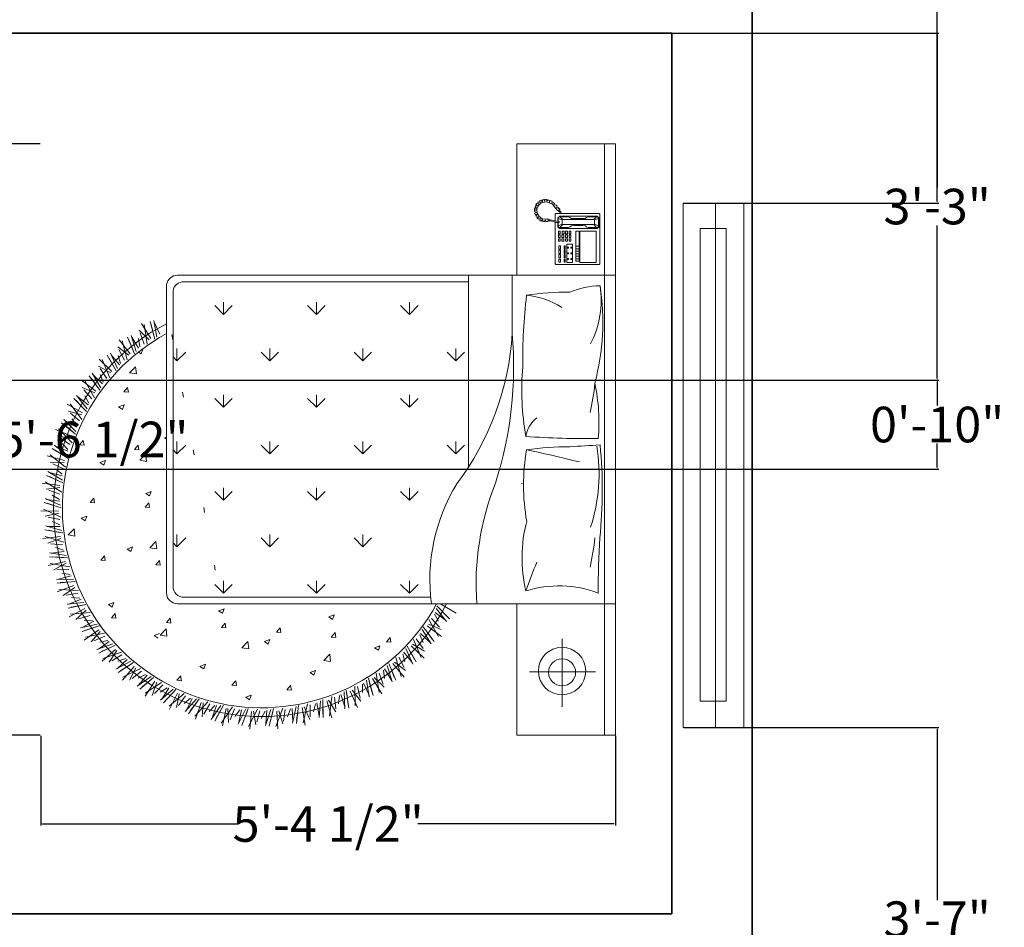
# Model space of a CAD drawing. Units: inches. Extents: x 311 to 754, y 60 to 497.
# Tile 8 of 11: x 641 to 751, y 194 to 296. Entities that reach past the tile are written whole.
import ezdxf

# ---------------------------------------------------------------- set-up
doc = ezdxf.new("R2010")
doc.units = ezdxf.units.IN
doc.header["$MEASUREMENT"] = 0
for name, color, linetype, lineweight in [('A-ANNO-DIMS', 2, 'Continuous', 18), ('A-WALL', 7, 'Continuous', 35), ('beds', 70, 'Continuous', 13), ('windows', 120, 'Continuous', 18)]:
    doc.layers.add(name, color=color, linetype=linetype, lineweight=lineweight)
doc.styles.get("Standard").update_dxf_attribs({"font": 'arial.ttf'})
doc.dimstyles.get("Standard").update_dxf_attribs({"dimtxt": 4, "dimasz": 0.18, "dimexe": 0.18, "dimexo": 0.0625, "dimgap": 0.09, "dimtad": 0, "dimtih": 1, "dimtoh": 1, "dimdec": 0, "dimrnd": 6, "dimzin": 0, "dimdsep": 46, "dimlunit": 3, "dimtxsty": 'Standard', "dimcen": 0.09, "dimadec": 0, "dimazin": 0, "dimtfac": 1, "dimtdec": 0, "dimtofl": 0, "dimtmove": 0, "dimatfit": 3, "dimfxl": 1, "dimtolj": 1, "dimtzin": 0, "dimarcsym": 0})

# ---------------------------------------------------------------- blocks, each defined once
blk = doc.blocks.new('A$C57792D97')
for p, q in [((0.6, 2.6235), (0, 2.6235)), ((0, 2.6235), (0, 2.1735)), ((2.1, 2.6235), (0.6, 2.6235)), ((0.6, 2.6235), (0.6, 0.6235)), ((0.6, 0.6235), (0.6, 2.6235)), ((0.6, 2.1735), (0.6, 2.6235)), ((2.1, 0.6235), (2.1, 2.6235)), ((2.7, 2.6235), (2.1, 2.6235)), ((2.1, 2.6235), (2.1, 2.1735)), ((2.7, 2.1735), (2.7, 2.6235)), ((0.6, 2.5735), (0, 2.5735)), ((2.1, 2.5735), (0.6, 2.5735)), ((2.7, 2.5735), (2.1, 2.5735)), ((2.4103, 2.2312), (2.4103, 2.5317)), ((2.2593, 2.3802), (2.5698, 2.3802)), ((0, 2.1735), (0.6, 2.1735)), ((1.5491, 2.1955), (1.5516, 2.1955)), ((2.1, 2.1735), (2.7, 2.1735)), ((0.6, 2.1518), (0.8661, 2.1518)), ((0.6, 1.9518), (1.4767, 1.9518)), ((0.63, 0.6535), (0.63, 1.9518)), ((0.9906, 1.8942), (0.9508, 1.934)), ((1.4149, 1.8942), (1.3751, 1.934)), ((0.9906, 1.8942), (0.9344, 1.8942)), ((0.9906, 1.8942), (0.9508, 1.8544)), ((1.4149, 1.8942), (1.3586, 1.8942)), ((1.4149, 1.8942), (1.3751, 1.8544)), ((2.142, 1.8959), (2.1018, 1.8254)), ((2.1679, 1.8652), (2.1088, 1.8077)), ((2.1584, 1.8544), (2.1201, 1.8188)), ((2.1812, 1.8524), (2.1207, 1.8046)), ((2.1749, 1.8475), (2.1394, 1.7993)), ((2.1799, 1.8155), (2.1465, 1.7971)), ((2.2066, 1.8191), (2.1664, 1.7827)), ((2.249, 1.8154), (2.1711, 1.7709)), ((2.2173, 1.8274), (2.1931, 1.7688)), ((2.2496, 1.8292), (2.2008, 1.7642)), ((2.07, 1.7793), (2.07, 0.6535)), ((2.2713, 1.7954), (2.2055, 1.7458)), ((2.283, 1.7811), (2.2169, 1.7413)), ((2.2607, 1.7859), (2.2181, 1.7554)), ((2.2761, 1.777), (2.2348, 1.7337)), ((0.7785, 1.6821), (0.7387, 1.7219)), ((1.2027, 1.6821), (1.163, 1.7219)), ((1.627, 1.6821), (1.5872, 1.7219)), ((2.0513, 1.6821), (2.0115, 1.7219)), ((2.277, 1.7446), (2.2416, 1.7306)), ((2.304, 1.7449), (2.2596, 1.7138)), ((2.3456, 1.7359), (2.2627, 1.7015)), ((2.3157, 1.7518), (2.2843, 1.6966)), ((2.3479, 1.7495), (2.2914, 1.6911)), ((2.3653, 1.7133), (2.2937, 1.6723)), ((0.7785, 1.6821), (0.7222, 1.6821)), ((0.7785, 1.6821), (0.7387, 1.6423)), ((1.2027, 1.6821), (1.1465, 1.6821)), ((1.2027, 1.6821), (1.163, 1.6423)), ((1.627, 1.6821), (1.5708, 1.6821)), ((1.627, 1.6821), (1.5872, 1.6423)), ((2.0513, 1.6821), (1.995, 1.6821)), ((2.0513, 1.6821), (2.0115, 1.6423)), ((2.3751, 1.6976), (2.3045, 1.6664)), ((2.3535, 1.7051), (2.3075, 1.6802)), ((2.3677, 1.6944), (2.3213, 1.6565)), ((2.4038, 1.6644), (2.3657, 1.6136)), ((2.3645, 1.6621), (2.3277, 1.6526)), ((2.3913, 1.659), (2.3434, 1.6337)), ((2.4314, 1.6449), (2.3449, 1.6211)), ((2.4355, 1.6581), (2.372, 1.6073)), ((2.4482, 1.62), (2.372, 1.5882)), ((2.2754, 1.598), (2.2534, 1.5939)), ((2.2736, 1.5771), (2.2535, 1.594)), ((2.2736, 1.5771), (2.2754, 1.598)), ((2.4559, 1.6032), (2.382, 1.581)), ((2.4354, 1.6134), (2.3867, 1.5944)), ((2.4482, 1.6009), (2.3974, 1.5692)), ((2.3123, 1.541), (2.2911, 1.5481)), ((2.3006, 1.5236), (2.2912, 1.5481)), ((2.3006, 1.5236), (2.3123, 1.541)), ((2.441, 1.5693), (2.4032, 1.5645)), ((2.4672, 1.5629), (2.4164, 1.5438)), ((2.5052, 1.5438), (2.4164, 1.5311)), ((2.4802, 1.5667), (2.4361, 1.5211)), ((2.5109, 1.5564), (2.4416, 1.514)), ((0.9906, 1.47), (0.9508, 1.5097)), ((1.4149, 1.47), (1.3751, 1.5097)), ((1.8391, 1.47), (1.7994, 1.5097)), ((2.5187, 1.517), (2.4392, 1.4951)), ((2.5243, 1.4994), (2.4482, 1.4867)), ((2.5052, 1.5121), (2.4545, 1.4994)), ((2.5163, 1.4981), (2.462, 1.473)), ((0.9906, 1.47), (0.9344, 1.47)), ((0.9906, 1.47), (0.9508, 1.4302)), ((1.4149, 1.47), (1.3586, 1.47)), ((1.4149, 1.47), (1.3751, 1.4302)), ((1.8391, 1.47), (1.7829, 1.47)), ((1.8391, 1.47), (1.7994, 1.4302)), ((2.5052, 1.4677), (2.4672, 1.4677)), ((2.5304, 1.458), (2.4777, 1.4454)), ((2.5438, 1.4601), (2.4943, 1.4204)), ((2.573, 1.4461), (2.4989, 1.4127)), ((2.5658, 1.4343), (2.4761, 1.4328)), ((2.5758, 1.406), (2.4942, 1.3942)), ((2.5618, 1.4028), (2.5099, 1.3966)), ((2.5791, 1.3878), (2.502, 1.3848)), ((2.571, 1.3876), (2.514, 1.3695)), ((2.5562, 1.3587), (2.5185, 1.3635)), ((2.1596, 1.3147), (2.1502, 1.3392)), ((2.1714, 1.3321), (2.1502, 1.3392)), ((2.1596, 1.3147), (2.1714, 1.3321)), ((2.2534, 1.3469), (2.2315, 1.3429)), ((2.2516, 1.326), (2.2315, 1.3429)), ((2.2516, 1.326), (2.2535, 1.347)), ((2.3632, 1.3229), (2.33, 1.319)), ((2.3584, 1.2918), (2.33, 1.319)), ((2.3584, 1.2918), (2.3632, 1.3229)), ((2.6121, 1.3181), (2.523, 1.3279)), ((2.58, 1.346), (2.5261, 1.3402)), ((2.5936, 1.3464), (2.5395, 1.3132)), ((2.6207, 1.3289), (2.5431, 1.305)), ((0.7785, 1.2578), (0.7387, 1.2976)), ((1.2027, 1.2578), (1.163, 1.2976)), ((1.627, 1.2578), (1.5872, 1.2976)), ((2.0513, 1.2578), (2.0115, 1.2976)), ((2.6185, 1.2888), (2.5361, 1.2873)), ((2.6195, 1.2703), (2.5426, 1.277)), ((2.6042, 1.2873), (2.5519, 1.2877)), ((2.6115, 1.2711), (2.5526, 1.2603)), ((0.7785, 1.2578), (0.7222, 1.2578)), ((0.7785, 1.2578), (0.7387, 1.218)), ((1.2027, 1.2578), (1.1465, 1.2578)), ((1.2027, 1.2578), (1.163, 1.218)), ((1.627, 1.2578), (1.5708, 1.2578)), ((1.627, 1.2578), (1.5872, 1.218)), ((2.0513, 1.2578), (1.995, 1.2578)), ((2.0513, 1.2578), (2.0115, 1.218)), ((2.4134, 1.2295), (2.404, 1.254)), ((2.4252, 1.2469), (2.404, 1.254)), ((2.4134, 1.2295), (2.4252, 1.2469)), ((2.5932, 1.2443), (2.5563, 1.2538)), ((2.6435, 1.197), (2.5563, 1.2178)), ((2.6152, 1.2287), (2.561, 1.2296)), ((2.6287, 1.2274), (2.5709, 1.2013)), ((2.6462, 1.1671), (2.5642, 1.176)), ((2.6534, 1.2066), (2.5734, 1.1926)), ((2.6319, 1.1675), (2.58, 1.1743)), ((2.4947, 1.1445), (2.4728, 1.1404)), ((2.4929, 1.1236), (2.4728, 1.1404)), ((2.4929, 1.1236), (2.4948, 1.1445)), ((2.6449, 1.1486), (2.5694, 1.1649)), ((2.637, 1.1504), (2.5773, 1.147)), ((2.6155, 1.1261), (2.5801, 1.1402)), ((0.9906, 1.0457), (0.9508, 1.0855)), ((1.4149, 1.0457), (1.3751, 1.0855)), ((1.8391, 1.0457), (1.7994, 1.0855)), ((2.2315, 1.0959), (2.2095, 1.0919)), ((2.2297, 1.075), (2.2096, 1.0919)), ((2.2297, 1.075), (2.2315, 1.0959)), ((2.6595, 1.0729), (2.5756, 1.1045)), ((2.6353, 1.1079), (2.5817, 1.1156)), ((2.6486, 1.1049), (2.588, 1.0862)), ((2.6705, 1.0812), (2.5894, 1.0774)), ((0.9906, 1.0457), (0.9344, 1.0457)), ((0.9906, 1.0457), (0.9508, 1.0059)), ((1.4149, 1.0457), (1.3586, 1.0457)), ((1.4149, 1.0457), (1.3751, 1.0059)), ((1.8391, 1.0457), (1.7829, 1.0457)), ((1.8391, 1.0457), (1.7994, 1.0059)), ((2.2725, 1.0206), (2.2631, 1.0451)), ((2.2842, 1.038), (2.2631, 1.0451)), ((2.2725, 1.0206), (2.2843, 1.038)), ((2.6584, 1.0429), (2.5782, 1.062)), ((2.6548, 1.0248), (2.582, 1.0503)), ((2.6442, 1.045), (2.5937, 1.0584)), ((2.6598, 0.9477), (2.5805, 0.9897)), ((2.6472, 1.0275), (2.5875, 1.0316)), ((2.6402, 0.9855), (2.588, 0.9999)), ((2.6228, 1.0061), (2.5895, 1.0244)), ((2.3053, 0.9493), (2.272, 0.9455)), ((2.3005, 0.9182), (2.2721, 0.9455)), ((2.3005, 0.9182), (2.3053, 0.9494)), ((2.5263, 0.9355), (2.5169, 0.96)), ((2.538, 0.9528), (2.5169, 0.9599)), ((2.5263, 0.9355), (2.5381, 0.9529)), ((2.655, 0.9181), (2.5778, 0.9471)), ((2.653, 0.9809), (2.5905, 0.97)), ((2.6718, 0.9546), (2.5908, 0.961)), ((2.6491, 0.9006), (2.5801, 0.9351)), ((2.6419, 0.9043), (2.5832, 0.9159)), ((2.6151, 0.8861), (2.5843, 0.9085)), ((2.6412, 0.9221), (2.5927, 0.9416)), ((0.7785, 0.8336), (0.7387, 0.8733)), ((1.2027, 0.8336), (1.163, 0.8733)), ((1.627, 0.8336), (1.5872, 0.8733)), ((2.0513, 0.8336), (2.0115, 0.8733)), ((2.4728, 0.8934), (2.4508, 0.8894)), ((2.471, 0.8725), (2.4509, 0.8894)), ((2.471, 0.8725), (2.4728, 0.8934)), ((2.6444, 0.8236), (2.571, 0.8751)), ((2.6418, 0.8573), (2.5785, 0.8543)), ((2.6297, 0.8635), (2.5797, 0.8843)), ((0.7785, 0.8336), (0.7222, 0.8336)), ((0.7785, 0.8336), (0.7387, 0.7938)), ((1.2027, 0.8336), (1.1465, 0.8336)), ((1.2027, 0.8336), (1.163, 0.7938)), ((1.627, 0.8336), (1.5708, 0.8336)), ((1.627, 0.8336), (1.5872, 0.7938)), ((2.0513, 0.8336), (1.995, 0.8336)), ((2.0513, 0.8336), (2.0115, 0.7938)), ((2.1316, 0.8117), (2.1222, 0.8362)), ((2.1433, 0.8291), (2.1222, 0.8362)), ((2.1316, 0.8117), (2.1434, 0.8291)), ((2.2095, 0.8449), (2.1876, 0.8408)), ((2.2077, 0.824), (2.1876, 0.8408)), ((2.2077, 0.824), (2.2095, 0.8449)), ((2.6359, 0.7948), (2.5629, 0.8332)), ((2.6279, 0.7781), (2.5637, 0.821)), ((2.6227, 0.8004), (2.577, 0.8259)), ((2.6572, 0.8289), (2.5776, 0.8454)), ((1.9462, 0.7963), (1.9243, 0.7923)), ((2.604, 0.7437), (2.557, 0.7707)), ((2.6212, 0.7827), (2.5644, 0.8015)), ((2.5923, 0.768), (2.5646, 0.7941)), ((1.683, 0.7477), (1.661, 0.7437)), ((2.3854, 0.7265), (2.376, 0.751)), ((2.3971, 0.7439), (2.376, 0.751)), ((2.3854, 0.7265), (2.3972, 0.7439)), ((2.6016, 0.6748), (2.534, 0.7221)), ((2.6136, 0.7023), (2.5472, 0.7626)), ((2.6269, 0.706), (2.5501, 0.7323)), ((2.6153, 0.7361), (2.552, 0.7411)), ((1.4197, 0.6992), (1.3978, 0.6951)), ((2.5549, 0.6537), (2.5307, 0.6831)), ((2.5855, 0.6646), (2.5315, 0.6905)), ((2.5915, 0.6593), (2.5332, 0.7099)), ((2.5892, 0.6821), (2.547, 0.7131)), ((0.9906, 0.6214), (0.9508, 0.6612)), ((1.1564, 0.6506), (1.1345, 0.6466)), ((1.4149, 0.6214), (1.3751, 0.6612)), ((1.8391, 0.6214), (1.7994, 0.6612)), ((2.4508, 0.6424), (2.4289, 0.6383)), ((2.449, 0.6215), (2.4289, 0.6384)), ((2.449, 0.6215), (2.4508, 0.6424)), ((2.5678, 0.5858), (2.5095, 0.654)), ((2.5737, 0.6192), (2.5116, 0.632)), ((2.5635, 0.6282), (2.5203, 0.6608)), ((2.02, 0.6035), (0.6716, 0.6035)), ((0.8932, 0.6021), (0.8712, 0.598)), ((0.9906, 0.6214), (0.9344, 0.6214)), ((0.9906, 0.6214), (0.9727, 0.6035)), ((1.4149, 0.6214), (1.3586, 0.6214)), ((1.4149, 0.6214), (1.397, 0.6035)), ((1.8391, 0.6214), (1.7829, 0.6214)), ((1.8391, 0.6214), (1.8212, 0.6035)), ((2.1875, 0.5938), (2.1656, 0.5898)), ((2.1857, 0.5729), (2.1656, 0.5898)), ((2.1857, 0.5729), (2.1876, 0.5938)), ((2.5352, 0.552), (2.4849, 0.5844)), ((2.5405, 0.546), (2.489, 0.6034)), ((2.5524, 0.5601), (2.4913, 0.6155)), ((2.541, 0.5688), (2.5031, 0.6049)), ((2.5815, 0.5878), (2.5085, 0.6236)), ((0.6417, 0.5735), (2.05, 0.5735)), ((0.8142, 0.5177), (0.8685, 0.5428)), ((1.3422, 0.5642), (1.3386, 0.5735)), ((1.3422, 0.5642), (1.3485, 0.5735)), ((1.9243, 0.5453), (1.9023, 0.5412)), ((1.9225, 0.5244), (1.9024, 0.5412)), ((1.9225, 0.5244), (1.9243, 0.5453)), ((2.2473, 0.5758), (2.2141, 0.5719)), ((2.2425, 0.5447), (2.2141, 0.572)), ((2.2445, 0.5176), (2.2351, 0.5421)), ((2.2425, 0.5447), (2.2474, 0.5758)), ((2.5078, 0.476), (2.4585, 0.551)), ((2.5088, 0.5186), (2.47, 0.5564)), ((2.5035, 0.545), (2.4831, 0.5772)), ((0.8062, 0.5164), (0.8823, 0.5291)), ((0.8118, 0.4988), (0.8913, 0.5207)), ((0.8196, 0.4594), (0.8889, 0.5018)), ((0.8253, 0.5037), (0.876, 0.5164)), ((0.8503, 0.4491), (0.8944, 0.4947)), ((1.6077, 0.4964), (1.5865, 0.5035)), ((1.596, 0.479), (1.5866, 0.5035)), ((1.596, 0.479), (1.6077, 0.4964)), ((1.661, 0.4967), (1.6391, 0.4927)), ((1.6592, 0.4758), (1.661, 0.4967)), ((1.8485, 0.5294), (1.8152, 0.5255)), ((1.8437, 0.4983), (1.8153, 0.5256)), ((1.8437, 0.4983), (1.8485, 0.5294)), ((2.2445, 0.5176), (2.2562, 0.535)), ((2.4757, 0.4399), (2.4318, 0.5034)), ((2.4893, 0.4525), (2.4356, 0.515)), ((2.4791, 0.4625), (2.446, 0.503)), ((2.5216, 0.4763), (2.4537, 0.5209)), ((2.5178, 0.5084), (2.4578, 0.5289)), ((0.8253, 0.472), (0.9141, 0.4847)), ((0.8633, 0.4529), (0.9141, 0.472)), ((0.8895, 0.4465), (0.9273, 0.4513)), ((0.9592, 0.4578), (0.938, 0.4649)), ((0.9403, 0.459), (0.9381, 0.4649)), ((0.9508, 0.4454), (0.9592, 0.4578)), ((1.4496, 0.483), (1.4163, 0.4791)), ((1.4448, 0.4519), (1.4164, 0.4792)), ((1.4448, 0.4519), (1.4496, 0.483)), ((1.6592, 0.4758), (1.6391, 0.4927)), ((2.4345, 0.3746), (2.395, 0.4552)), ((2.4409, 0.4167), (2.4071, 0.4591)), ((2.4389, 0.4436), (2.4227, 0.478)), ((2.4712, 0.4466), (2.4253, 0.485)), ((0.8746, 0.4126), (0.9485, 0.4347)), ((0.8823, 0.4149), (0.9331, 0.4466)), ((0.8823, 0.3958), (0.9585, 0.4275)), ((0.895, 0.3577), (0.9585, 0.4085)), ((0.8951, 0.4024), (0.9438, 0.4214)), ((1.0507, 0.4366), (1.0175, 0.4327)), ((1.0459, 0.4055), (1.0175, 0.4328)), ((1.0459, 0.4055), (1.0507, 0.4366)), ((1.3977, 0.4481), (1.3758, 0.4441)), ((1.3959, 0.4272), (1.3758, 0.4441)), ((1.3959, 0.4272), (1.3978, 0.4482)), ((1.8615, 0.4113), (1.8403, 0.4184)), ((1.8498, 0.3939), (1.8404, 0.4184)), ((1.8498, 0.3939), (1.8615, 0.4113)), ((2.3981, 0.3428), (2.3625, 0.4113)), ((2.4132, 0.3535), (2.3678, 0.4224)), ((2.4043, 0.3648), (2.3766, 0.4092)), ((2.4482, 0.3731), (2.3865, 0.4259)), ((2.4485, 0.4055), (2.3915, 0.4334)), ((0.8991, 0.3709), (0.9856, 0.3946)), ((0.9267, 0.3514), (0.9648, 0.4022)), ((0.9392, 0.3568), (0.9872, 0.3821)), ((0.966, 0.3537), (1.0029, 0.3631)), ((1.1345, 0.3996), (1.1125, 0.3955)), ((1.1327, 0.3787), (1.1126, 0.3955)), ((1.1327, 0.3787), (1.1345, 0.3996)), ((1.213, 0.3727), (1.1918, 0.3798)), ((1.2013, 0.3553), (1.1919, 0.3798)), ((1.2013, 0.3553), (1.213, 0.3727)), ((2.3491, 0.2832), (2.32, 0.3681)), ((2.3607, 0.3242), (2.3324, 0.3704)), ((2.3621, 0.3511), (2.3503, 0.3873)), ((2.3945, 0.35), (2.3538, 0.3939)), ((0.9555, 0.3182), (1.026, 0.3494)), ((0.9628, 0.3214), (1.0092, 0.3592)), ((0.9652, 0.3025), (1.0368, 0.3435)), ((0.977, 0.3107), (1.023, 0.3356)), ((0.9826, 0.2663), (1.0392, 0.3246)), ((1.0148, 0.264), (1.0462, 0.3191)), ((2.1153, 0.3261), (2.0941, 0.3332)), ((2.1036, 0.3087), (2.0942, 0.3332)), ((2.1036, 0.3087), (2.1153, 0.3261)), ((2.1656, 0.3428), (2.1436, 0.3387)), ((2.1638, 0.3219), (2.1437, 0.3388)), ((2.1638, 0.3219), (2.1656, 0.3428)), ((2.309, 0.2562), (2.2823, 0.3286)), ((2.3253, 0.265), (2.2888, 0.3389)), ((2.3179, 0.2773), (2.2959, 0.3247)), ((2.3625, 0.28), (2.3078, 0.3401)), ((2.3668, 0.3121), (2.3138, 0.3469)), ((0.9849, 0.2799), (1.0678, 0.3143)), ((1.0265, 0.2709), (1.0709, 0.302)), ((1.0475, 0.2347), (1.1136, 0.2745)), ((1.0535, 0.2712), (1.0889, 0.2852)), ((1.0544, 0.2388), (1.0957, 0.2821)), ((1.0592, 0.2203), (1.125, 0.27)), ((1.4668, 0.2875), (1.4456, 0.2946)), ((1.4551, 0.2701), (1.4457, 0.2946)), ((1.4551, 0.2701), (1.4668, 0.2875)), ((1.9023, 0.2942), (1.8804, 0.2902)), ((1.9005, 0.2733), (1.8804, 0.2902)), ((1.9005, 0.2733), (1.9023, 0.2942)), ((2.2741, 0.2296), (2.2258, 0.2708)), ((2.2529, 0.2032), (2.2346, 0.291)), ((2.2695, 0.2424), (2.2473, 0.2918)), ((2.2743, 0.2689), (2.2671, 0.3063)), ((2.3063, 0.2638), (2.2714, 0.3124)), ((1.0699, 0.2299), (1.1124, 0.2604)), ((1.0809, 0.1866), (1.1297, 0.2516)), ((1.0815, 0.2004), (1.1594, 0.2449)), ((1.1132, 0.1884), (1.1374, 0.247)), ((1.1239, 0.1967), (1.1641, 0.2331)), ((1.639, 0.2457), (1.6171, 0.2416)), ((1.6372, 0.2248), (1.6171, 0.2416)), ((1.6372, 0.2248), (1.6391, 0.2457)), ((2.1474, 0.1359), (2.1403, 0.2253)), ((2.1768, 0.1984), (2.1745, 0.2364)), ((2.208, 0.1893), (2.1795, 0.2419)), ((2.2097, 0.1814), (2.1923, 0.2566)), ((2.227, 0.1881), (2.2001, 0.2661)), ((2.2212, 0.2012), (2.2053, 0.2511)), ((2.2658, 0.1984), (2.2191, 0.2649)), ((1.1493, 0.1634), (1.2098, 0.2112)), ((1.1507, 0.2003), (1.184, 0.2187)), ((1.1556, 0.1683), (1.1911, 0.2165)), ((1.1626, 0.1506), (1.2217, 0.2081)), ((1.1721, 0.1614), (1.2104, 0.197)), ((1.1873, 0.1336), (1.259, 0.1875)), ((1.1885, 0.1199), (1.2287, 0.1904)), ((1.2203, 0.1256), (1.237, 0.1868)), ((1.3758, 0.1971), (1.3538, 0.193)), ((1.374, 0.1762), (1.3539, 0.1931)), ((1.374, 0.1762), (1.3758, 0.1971)), ((1.7206, 0.2023), (1.6994, 0.2094)), ((1.7089, 0.1849), (1.6995, 0.2095)), ((1.7089, 0.1849), (1.7206, 0.2024)), ((2.1011, 0.1277), (2.0794, 0.1835)), ((2.1018, 0.1197), (2.0939, 0.1965)), ((2.1198, 0.1242), (2.1029, 0.2049)), ((2.1157, 0.1379), (2.1062, 0.1893)), ((2.1596, 0.1295), (2.1216, 0.2013)), ((2.1718, 0.1594), (2.129, 0.2063)), ((2.1688, 0.1727), (2.1529, 0.2245)), ((1.2299, 0.1352), (1.2652, 0.1764)), ((1.2559, 0.1422), (1.2867, 0.1646)), ((1.2592, 0.1054), (1.3133, 0.1604)), ((1.2649, 0.111), (1.2941, 0.1633)), ((1.2741, 0.0944), (1.3255, 0.1588)), ((1.282, 0.1063), (1.3156, 0.1464)), ((1.3007, 0.0806), (1.3651, 0.1431)), ((1.3035, 0.0671), (1.3346, 0.1421)), ((1.3344, 0.0768), (1.3433, 0.1396)), ((1.7905, 0.1559), (1.7573, 0.152)), ((1.7857, 0.1248), (1.7573, 0.152)), ((1.7857, 0.1248), (1.7906, 0.1559)), ((1.9873, 0.08), (1.9728, 0.1381)), ((1.9871, 0.072), (1.9889, 0.1491)), ((2.0054, 0.0742), (1.9988, 0.1564)), ((2.0031, 0.0883), (2.0001, 0.1405)), ((2.0456, 0.0745), (2.0169, 0.1505)), ((2.0614, 0.1027), (2.0249, 0.1545)), ((2.0343, 0.0824), (2.0385, 0.172)), ((2.0601, 0.1162), (2.0509, 0.1696)), ((2.0714, 0.1407), (2.0737, 0.1787)), ((1.3427, 0.0876), (1.3725, 0.1328)), ((1.3677, 0.0977), (1.3954, 0.1238)), ((1.3755, 0.0616), (1.4223, 0.1229)), ((1.3804, 0.0679), (1.4028, 0.1234)), ((1.3916, 0.0525), (1.4346, 0.1229)), ((1.3981, 0.0653), (1.4264, 0.1093)), ((1.4198, 0.0422), (1.4758, 0.1123)), ((1.4243, 0.0292), (1.4458, 0.1075)), ((1.4537, 0.0427), (1.4546, 0.1061)), ((1.4606, 0.0544), (1.4845, 0.103)), ((1.4841, 0.0676), (1.5083, 0.0969)), ((1.4964, 0.0327), (1.5351, 0.0995)), ((1.5005, 0.0397), (1.5158, 0.0975)), ((1.5135, 0.0258), (1.5473, 0.101)), ((1.5428, 0.0191), (1.5896, 0.0956)), ((1.6199, 0.0192), (1.65, 0.0903)), ((1.6378, 0.0145), (1.6619, 0.0934)), ((1.6677, 0.0115), (1.7045, 0.0933)), ((1.7442, 0.0214), (1.7651, 0.0956)), ((1.7625, 0.0189), (1.7765, 0.1002)), ((1.7925, 0.0197), (1.8188, 0.1054)), ((1.8015, 0.0092), (1.7926, 0.09)), ((1.8238, 0.0326), (1.8014, 0.0919)), ((1.8259, 0.046), (1.8303, 0.1)), ((1.8429, 0.0669), (1.8547, 0.1031)), ((1.8685, 0.047), (1.8614, 0.1064)), ((1.8672, 0.039), (1.8787, 0.1154)), ((1.8852, 0.0532), (1.8888, 0.1054)), ((1.8857, 0.0389), (1.8894, 0.1213)), ((1.9256, 0.0342), (1.9067, 0.1132)), ((1.9448, 0.0601), (1.9151, 0.1162)), ((1.9154, 0.0434), (1.9307, 0.1318)), ((1.9452, 0.0737), (1.9428, 0.1279)), ((1.9595, 0.0966), (1.9666, 0.134)), ((1.5183, 0.0393), (1.5409, 0.0865)), ((1.5489, 0.0067), (1.5603, 0.0871)), ((1.5763, 0.0238), (1.5693, 0.0868)), ((1.5817, 0.0362), (1.5994, 0.0875)), ((1.6034, 0.0523), (1.6237, 0.0845)), ((1.6232, 0.0266), (1.631, 0.086)), ((1.6409, 0.0285), (1.6573, 0.0782)), ((1.6753, 0), (1.6766, 0.0812)), ((1.7004, 0.0204), (1.6855, 0.0821)), ((1.7041, 0.0334), (1.7152, 0.0865)), ((1.7236, 0.0521), (1.7398, 0.0865)), ((1.7465, 0.0291), (1.7469, 0.0889)), ((1.7638, 0.0332), (1.7739, 0.0845))]:
    blk.add_line(p, q)
at = {"linetype": 'ByBlock'}
for p, q in [((0.3217, 2.5511), (0.3189, 2.5483)), ((0.3189, 2.5483), (0.3189, 2.3511)), ((0.5475, 2.5511), (0.3217, 2.5511)), ((0.3375, 2.5469), (0.3303, 2.5397)), ((0.3303, 2.5397), (0.3303, 2.3683)), ((0.3346, 2.5426), (0.3332, 2.5369)), ((0.3332, 2.5369), (0.3332, 2.4983)), ((0.3332, 2.5369), (0.346, 2.524)), ((0.3403, 2.5454), (0.3346, 2.5426)), ((0.3803, 2.5469), (0.3375, 2.5469)), ((0.3746, 2.5454), (0.3403, 2.5454)), ((0.3475, 2.5269), (0.3403, 2.5454)), ((0.346, 2.524), (0.3475, 2.5269)), ((0.346, 2.4597), (0.346, 2.524)), ((0.3475, 2.5269), (0.3675, 2.5269)), ((0.3675, 2.5269), (0.3746, 2.5454)), ((0.3689, 2.524), (0.3675, 2.5269)), ((0.3818, 2.5369), (0.3689, 2.524)), ((0.3689, 2.4597), (0.3689, 2.524)), ((0.3746, 2.5454), (0.3803, 2.5426)), ((0.386, 2.5397), (0.3803, 2.5469)), ((0.3803, 2.5426), (0.3818, 2.5369)), ((0.3818, 2.5369), (0.3818, 2.4983)), ((0.386, 2.3668), (0.386, 2.5397)), ((0.3989, 2.4597), (0.3989, 2.5354)), ((0.3989, 2.5354), (0.5418, 2.5354)), ((0.5418, 2.5354), (0.5418, 2.4597)), ((0.5475, 2.5511), (0.5503, 2.5483)), ((0.5503, 2.5483), (0.5503, 2.3511)), ((0.3332, 2.4983), (0.336, 2.4911)), ((0.336, 2.4911), (0.3403, 2.484)), ((0.3403, 2.484), (0.3417, 2.474)), ((0.3417, 2.474), (0.3417, 2.4597)), ((0.3746, 2.484), (0.3732, 2.474)), ((0.3732, 2.474), (0.3732, 2.4597)), ((0.3789, 2.4911), (0.3746, 2.484)), ((0.3818, 2.4983), (0.3789, 2.4911)), ((0.3403, 2.4226), (0.3417, 2.4326)), ((0.3417, 2.4326), (0.3417, 2.4597)), ((0.346, 2.4597), (0.346, 2.3826)), ((0.3689, 2.4597), (0.3689, 2.3826)), ((0.3732, 2.4326), (0.3732, 2.4597)), ((0.3746, 2.4226), (0.3732, 2.4326)), ((0.5418, 2.4597), (0.3989, 2.4597)), ((0.3989, 2.4426), (0.3989, 2.4568)), ((0.3989, 2.4568), (0.5361, 2.4568)), ((0.5361, 2.4426), (0.3989, 2.4426)), ((0.4675, 2.4568), (0.4675, 2.4426)), ((0.4789, 2.4568), (0.4789, 2.4426)), ((0.4903, 2.4568), (0.4903, 2.4426)), ((0.5018, 2.4568), (0.5018, 2.4426)), ((0.5132, 2.4568), (0.5132, 2.4426)), ((0.5246, 2.4568), (0.5246, 2.4426)), ((0.5361, 2.4568), (0.5361, 2.4426)), ((0.3332, 2.4083), (0.336, 2.4154)), ((0.3332, 2.3697), (0.3332, 2.4083)), ((0.3332, 2.3697), (0.346, 2.3826)), ((0.336, 2.4154), (0.3403, 2.4226)), ((0.346, 2.3826), (0.3475, 2.3797)), ((0.3689, 2.3826), (0.3675, 2.3797)), ((0.3818, 2.3697), (0.3689, 2.3826)), ((0.3789, 2.4154), (0.3746, 2.4226)), ((0.3818, 2.4083), (0.3789, 2.4154)), ((0.3818, 2.3697), (0.3818, 2.4083)), ((0.3989, 2.4197), (0.3989, 2.4111)), ((0.4103, 2.4197), (0.3989, 2.4197)), ((0.3989, 2.4111), (0.4103, 2.4111)), ((0.3989, 2.404), (0.3989, 2.3954)), ((0.4103, 2.404), (0.3989, 2.404)), ((0.3989, 2.3954), (0.4103, 2.3954)), ((0.4103, 2.3883), (0.3989, 2.3883)), ((0.3989, 2.3883), (0.3989, 2.3797)), ((0.4103, 2.4111), (0.4103, 2.4197)), ((0.4103, 2.3954), (0.4103, 2.404)), ((0.4103, 2.3797), (0.4103, 2.3883)), ((0.4275, 2.4197), (0.416, 2.4197)), ((0.416, 2.4197), (0.416, 2.4111)), ((0.416, 2.4111), (0.4275, 2.4111)), ((0.416, 2.404), (0.416, 2.3954)), ((0.4275, 2.404), (0.416, 2.404)), ((0.416, 2.3954), (0.4275, 2.3954)), ((0.4275, 2.3868), (0.416, 2.3868)), ((0.416, 2.3868), (0.416, 2.3783)), ((0.4275, 2.4111), (0.4275, 2.4197)), ((0.4275, 2.3954), (0.4275, 2.404)), ((0.4275, 2.3783), (0.4275, 2.3868)), ((0.4332, 2.4197), (0.4332, 2.4111)), ((0.4446, 2.4197), (0.4332, 2.4197)), ((0.4332, 2.4111), (0.4446, 2.4111)), ((0.4332, 2.404), (0.4332, 2.3954)), ((0.4446, 2.404), (0.4332, 2.404)), ((0.4332, 2.3954), (0.4446, 2.3954)), ((0.4446, 2.3868), (0.4332, 2.3868)), ((0.4332, 2.3868), (0.4332, 2.3783)), ((0.4446, 2.4111), (0.4446, 2.4197)), ((0.4446, 2.3954), (0.4446, 2.404)), ((0.4446, 2.3783), (0.4446, 2.3868)), ((0.4575, 2.4011), (0.4575, 2.4268)), ((0.4575, 2.4268), (0.5418, 2.4268)), ((0.5418, 2.4011), (0.4575, 2.4011)), ((0.4661, 2.394), (0.4803, 2.394)), ((0.4661, 2.3883), (0.4661, 2.394)), ((0.4803, 2.3883), (0.4661, 2.3883)), ((0.4718, 2.424), (0.4761, 2.424)), ((0.4718, 2.4197), (0.4718, 2.424)), ((0.4761, 2.4197), (0.4718, 2.4197)), ((0.4718, 2.4083), (0.4761, 2.4083)), ((0.4718, 2.404), (0.4718, 2.4083)), ((0.4761, 2.404), (0.4718, 2.404)), ((0.4761, 2.424), (0.4761, 2.4197)), ((0.4761, 2.4083), (0.4761, 2.404)), ((0.4803, 2.394), (0.4803, 2.3883)), ((0.4861, 2.3883), (0.4861, 2.394)), ((0.4861, 2.394), (0.5003, 2.394)), ((0.5003, 2.3883), (0.4861, 2.3883)), ((0.4975, 2.424), (0.5018, 2.424)), ((0.4975, 2.4197), (0.4975, 2.424)), ((0.5018, 2.4197), (0.4975, 2.4197)), ((0.4975, 2.4083), (0.5018, 2.4083)), ((0.4975, 2.404), (0.4975, 2.4083)), ((0.5018, 2.404), (0.4975, 2.404)), ((0.5003, 2.394), (0.5003, 2.3883)), ((0.5018, 2.424), (0.5018, 2.4197)), ((0.5018, 2.4083), (0.5018, 2.404)), ((0.5061, 2.3883), (0.5061, 2.394)), ((0.5061, 2.394), (0.5203, 2.394)), ((0.5203, 2.3883), (0.5061, 2.3883)), ((0.5203, 2.394), (0.5203, 2.3883)), ((0.5232, 2.4197), (0.5232, 2.424)), ((0.5232, 2.424), (0.5275, 2.424)), ((0.5275, 2.4197), (0.5232, 2.4197)), ((0.5232, 2.4083), (0.5275, 2.4083)), ((0.5232, 2.404), (0.5232, 2.4083)), ((0.5275, 2.404), (0.5232, 2.404)), ((0.5261, 2.3883), (0.5261, 2.394)), ((0.5261, 2.394), (0.5403, 2.394)), ((0.5403, 2.3883), (0.5261, 2.3883)), ((0.5275, 2.424), (0.5275, 2.4197)), ((0.5275, 2.4083), (0.5275, 2.404)), ((0.5403, 2.394), (0.5403, 2.3883)), ((0.5418, 2.4268), (0.5418, 2.4011)), ((0.2683, 2.3394), (0.2738, 2.3452)), ((0.2706, 2.3331), (0.2683, 2.3394)), ((0.2738, 2.3452), (0.2804, 2.3412)), ((0.2937, 2.3497), (0.2748, 2.3336)), ((0.2789, 2.3502), (0.2854, 2.3565)), ((0.2804, 2.3412), (0.2789, 2.3502)), ((0.2854, 2.3565), (0.2932, 2.3525)), ((0.2902, 2.3608), (0.294, 2.3648)), ((0.2932, 2.3525), (0.2902, 2.3608)), ((0.3053, 2.3601), (0.2937, 2.3497)), ((0.294, 2.3648), (0.2975, 2.3621)), ((0.2955, 2.3663), (0.298, 2.3689)), ((0.2975, 2.3621), (0.2955, 2.3663)), ((0.298, 2.3689), (0.3033, 2.3669)), ((0.3053, 2.3628), (0.3023, 2.3631)), ((0.3023, 2.3631), (0.3053, 2.3601)), ((0.3033, 2.3669), (0.3063, 2.3696)), ((0.3068, 2.3648), (0.3053, 2.3628)), ((0.3063, 2.3696), (0.3103, 2.3737)), ((0.3126, 2.3694), (0.3068, 2.3648)), ((0.3103, 2.3737), (0.3189, 2.3768)), ((0.3189, 2.3711), (0.3126, 2.3694)), ((0.3189, 2.3511), (0.3217, 2.3483)), ((0.3217, 2.3483), (0.3525, 2.3483)), ((0.3303, 2.3683), (0.3375, 2.3597)), ((0.3346, 2.364), (0.3332, 2.3697)), ((0.3403, 2.3611), (0.3346, 2.364)), ((0.3375, 2.3597), (0.3542, 2.3597)), ((0.3475, 2.3797), (0.3403, 2.3611)), ((0.3543, 2.3611), (0.3403, 2.3611)), ((0.3475, 2.3797), (0.3675, 2.3797)), ((0.3483, 2.3311), (0.3518, 2.3447)), ((0.3518, 2.3447), (0.3538, 2.354)), ((0.3552, 2.3386), (0.3518, 2.325)), ((0.3538, 2.354), (0.3546, 2.3654)), ((0.3546, 2.3654), (0.3589, 2.3654)), ((0.3587, 2.3531), (0.3552, 2.3386)), ((0.3575, 2.3483), (0.5475, 2.3483)), ((0.3589, 2.3654), (0.3587, 2.3531)), ((0.3746, 2.3611), (0.3588, 2.3611)), ((0.3588, 2.3597), (0.3789, 2.3597)), ((0.3675, 2.3797), (0.3746, 2.3611)), ((0.3746, 2.3611), (0.3803, 2.364)), ((0.3789, 2.3597), (0.386, 2.3668)), ((0.3803, 2.364), (0.3818, 2.3697)), ((0.3989, 2.3797), (0.4103, 2.3797)), ((0.4103, 2.3711), (0.3989, 2.3711)), ((0.3989, 2.3711), (0.3989, 2.3626)), ((0.3989, 2.3626), (0.4103, 2.3626)), ((0.4103, 2.3626), (0.4103, 2.3711)), ((0.416, 2.3783), (0.4275, 2.3783)), ((0.416, 2.3711), (0.416, 2.3626)), ((0.4275, 2.3711), (0.416, 2.3711)), ((0.416, 2.3626), (0.4275, 2.3626)), ((0.4275, 2.3626), (0.4275, 2.3711)), ((0.4332, 2.3783), (0.4446, 2.3783)), ((0.4332, 2.3711), (0.4332, 2.3626)), ((0.4446, 2.3711), (0.4332, 2.3711)), ((0.4332, 2.3626), (0.4446, 2.3626)), ((0.4446, 2.3626), (0.4446, 2.3711)), ((0.4661, 2.3726), (0.4661, 2.364)), ((0.4803, 2.3726), (0.4661, 2.3726)), ((0.4661, 2.364), (0.4803, 2.364)), ((0.4803, 2.364), (0.4803, 2.3726)), ((0.5003, 2.3726), (0.4861, 2.3726)), ((0.4861, 2.3726), (0.4861, 2.364)), ((0.4861, 2.364), (0.5003, 2.364)), ((0.5003, 2.364), (0.5003, 2.3726)), ((0.5203, 2.3726), (0.5061, 2.3726)), ((0.5061, 2.3726), (0.5061, 2.364)), ((0.5061, 2.364), (0.5203, 2.364)), ((0.5203, 2.364), (0.5203, 2.3726)), ((0.5403, 2.3726), (0.5261, 2.3726)), ((0.5261, 2.3726), (0.5261, 2.364)), ((0.5261, 2.364), (0.5403, 2.364)), ((0.5403, 2.364), (0.5403, 2.3726)), ((0.5503, 2.3511), (0.5475, 2.3483)), ((0.2532, 2.3027), (0.2546, 2.31)), ((0.2621, 2.3001), (0.2532, 2.3027)), ((0.2546, 2.31), (0.2624, 2.31)), ((0.2546, 2.2958), (0.2621, 2.3001)), ((0.2558, 2.29), (0.2546, 2.2958)), ((0.2563, 2.3158), (0.2584, 2.3224)), ((0.2624, 2.31), (0.2563, 2.3158)), ((0.2584, 2.3224), (0.2676, 2.3221)), ((0.2592, 2.3253), (0.2618, 2.334)), ((0.2676, 2.3221), (0.2592, 2.3253)), ((0.2618, 2.334), (0.2705, 2.3331)), ((0.2746, 2.3331), (0.265, 2.3059)), ((0.265, 2.3059), (0.2691, 2.2842)), ((0.3422, 2.288), (0.3437, 2.3062)), ((0.3425, 2.3129), (0.3477, 2.3166)), ((0.3437, 2.3062), (0.3425, 2.3129)), ((0.3549, 2.3056), (0.3466, 2.3042)), ((0.3466, 2.3042), (0.3546, 2.2993)), ((0.3474, 2.3242), (0.3483, 2.3311)), ((0.3477, 2.3166), (0.3474, 2.3242)), ((0.352, 2.3175), (0.3512, 2.3158)), ((0.3512, 2.3158), (0.3544, 2.3126)), ((0.3518, 2.325), (0.352, 2.3175)), ((0.3546, 2.2993), (0.3541, 2.2915)), ((0.3544, 2.3126), (0.3549, 2.3056)), ((0.2647, 2.2903), (0.2558, 2.29)), ((0.2578, 2.2825), (0.2647, 2.2903)), ((0.2601, 2.2767), (0.2578, 2.2825)), ((0.2685, 2.2793), (0.2601, 2.2767)), ((0.2644, 2.2715), (0.2685, 2.2793)), ((0.2682, 2.268), (0.2644, 2.2715)), ((0.2763, 2.2715), (0.2682, 2.268)), ((0.2691, 2.2842), (0.2818, 2.2718)), ((0.2728, 2.2637), (0.2763, 2.2715)), ((0.2774, 2.2596), (0.2728, 2.2637)), ((0.2835, 2.2672), (0.2774, 2.2596)), ((0.2818, 2.2718), (0.2986, 2.2646)), ((0.2827, 2.2585), (0.2835, 2.2672)), ((0.2873, 2.2562), (0.2827, 2.2585)), ((0.2939, 2.262), (0.2873, 2.2562)), ((0.2942, 2.2541), (0.2939, 2.262)), ((0.2997, 2.2527), (0.2942, 2.2541)), ((0.2986, 2.2646), (0.3159, 2.266)), ((0.3029, 2.262), (0.2997, 2.2527)), ((0.3049, 2.2536), (0.3029, 2.262)), ((0.3098, 2.2541), (0.3049, 2.2536)), ((0.3133, 2.262), (0.3098, 2.2541)), ((0.3171, 2.2541), (0.3133, 2.262)), ((0.3159, 2.266), (0.3312, 2.2741)), ((0.3231, 2.2559), (0.3171, 2.2541)), ((0.3292, 2.2596), (0.3223, 2.2654)), ((0.3223, 2.2654), (0.3231, 2.2559)), ((0.3347, 2.2631), (0.3292, 2.2596)), ((0.3312, 2.2741), (0.3422, 2.288)), ((0.3402, 2.266), (0.3335, 2.2709)), ((0.3335, 2.2709), (0.3347, 2.2631)), ((0.3445, 2.2712), (0.3402, 2.266)), ((0.3492, 2.2776), (0.3405, 2.2793)), ((0.3405, 2.2793), (0.3445, 2.2712)), ((0.3541, 2.2915), (0.3448, 2.2906)), ((0.3448, 2.2906), (0.3529, 2.2842)), ((0.3529, 2.2842), (0.3492, 2.2776))]:
    blk.add_line(p, q, dxfattribs=at)
for centre, radius in [((2.4068, 2.3792), 0.1082), ((2.4128, 2.3792), 0.062)]:
    blk.add_circle(centre, radius)
for centre, radius, start, end in [((0.8117, 1.4495), 1.1155, 75.3755, 98.4519), ((1.5803, 0.4369), 2.1259, 84.0997, 95.547), ((0.7133, 2.123), 0.4349, 62.6153, 98.6623), ((0.9995, 2.5566), 0.3518, 180.6066, 203.849), ((1.2711, 1.6927), 0.8548, 85.0132, 101.9962), ((0.9942, 1.5092), 1.0245, 76.8495, 84.445), ((-2.6554, 2.4937), 4.0011, 355.9906, 0.7251), ((7.229, 2.8402), 5.8612, 182.80995, 184.16642), ((1.505, 1.754), 0.7941, 71.9705, 99.0452), ((2.0384, 6.4739), 3.9297, 266.5056, 270.1818), ((1.6997, 1.5092), 1.0245, 76.8495, 84.445), ((2.5231, 2.3654), 0.505, 159.2551, 197.4606), ((6.5168, 1.1676), 5.2262, 165.6998, 168.4122), ((1.7461, 2.3905), 1.0686, 178.7205, 189.3246), ((2.4516, 2.3905), 1.0686, 178.7205, 189.3246), ((1.0382, 2.187), 0.3479, 146.8128, 174.9884), ((1.3553, 2.3447), 0.1322, 217.4973, 261.5591), ((2.6076, 3.8927), 1.7717, 246.8027, 251.3608), ((0.9964, 4.7934), 2.5939, 263.2521, 270.4789), ((1.1218, 3.4256), 1.2305, 265.1643, 280.0187), ((1.5587, 3.1365), 0.9332, 260.0314, 280.1788), ((1.8907, 2.8521), 0.6558, 255.2386, 283.2855), ((1.0153, 0.392), 1.7661, 72.4208, 94.846), ((0.7898, 0.8867), 1.2674, 53.0057, 86.5496), ((2.0108, 3.233), 1.2462, 248.2311, 274.1028), ((1.991, 2.6169), 0.8413, 238.5747, 277.4412), ((1.6653, 1.0079), 0.9493, 207.2312, 62.7432), ((1.6653, 1.0079), 0.9093, 208.5361, 61.4369), ((0.6787, 0.6517), 0.0487, 177.8916, 261.664), ((2.02, 0.6535), 0.05, 270, 0), ((0.6518, 0.6244), 0.0518, 180.9151, 258.7324), ((2.05, 0.6235), 0.05, 270, 0)]:
    blk.add_arc(centre, radius, start, end)
blk = doc.blocks.new('WIN-FRAME-59IN')
for points in [[(0, 0), (0, 6.8), (58.92, 6.8), (58.92, 0)], [(2.85, 4.84), (55.97, 4.84), (55.97, 1.89), (2.85, 1.89)]]:
    blk.add_lwpolyline(points, close=True)
blk = doc.blocks.new('*D108')
at = {"layer": 'A-ANNO-DIMS', "color": 0, "lineweight": -2, "transparency": 16777216}
for p, q in [((642.81, 281.79), (632.73, 281.79)), ((632.91, 281.61), (632.91, 250.72)), ((632.91, 215.5), (632.91, 246.4)), ((642.81, 215.32), (632.73, 215.32))]:
    blk.add_line(p, q, dxfattribs=at)
at = {"layer": 'A-ANNO-DIMS', "color": 0, "transparency": 16777216}
for points in [[(632.88, 281.61), (632.94, 281.61), (632.91, 281.79)], [(632.88, 215.5), (632.94, 215.5), (632.91, 215.32)]]:
    blk.add_solid(points, dxfattribs=at)
at = {"layer": 'Defpoints', "color": 0, "transparency": 16777216}
for p in [(642.88, 281.79), (632.91, 215.32), (642.88, 215.32)]:
    blk.add_point(p, dxfattribs=at)
at = {"layer": 'A-ANNO-DIMS', "color": 0, "transparency": 16777216, "insert": (632.91, 248.56), "char_height": 4, "attachment_point": 5}
blk.add_mtext('\\A1;BED GROUP 5\'-6 1/2"', dxfattribs=at)
blk = doc.blocks.new('*D109')
at = {"layer": 'A-ANNO-DIMS', "color": 0, "lineweight": -2, "transparency": 16777216}
for p, q in [((642.88, 215.26), (642.88, 205.17)), ((707.46, 215.26), (707.46, 205.17)), ((643.06, 205.35), (665.1, 205.35)), ((707.28, 205.35), (685.24, 205.35))]:
    blk.add_line(p, q, dxfattribs=at)
at = {"layer": 'A-ANNO-DIMS', "color": 0, "transparency": 16777216}
for points in [[(643.06, 205.38), (643.06, 205.32), (642.88, 205.35)], [(707.28, 205.38), (707.28, 205.32), (707.46, 205.35)]]:
    blk.add_solid(points, dxfattribs=at)
at = {"layer": 'Defpoints', "color": 0, "transparency": 16777216}
for p in [(642.88, 215.32), (707.46, 215.32), (707.46, 205.35)]:
    blk.add_point(p, dxfattribs=at)
at = {"layer": 'A-ANNO-DIMS', "color": 0, "transparency": 16777216, "insert": (675.17, 205.35), "char_height": 4, "attachment_point": 5}
blk.add_mtext('\\A1;5\'-4 1/2"', dxfattribs=at)
blk = doc.blocks.new('*D122')
at = {"layer": 'A-ANNO-DIMS', "color": 0, "lineweight": -2, "transparency": 16777216}
for p, q in [((715.2, 358.24), (743.78, 358.24)), ((743.6, 358.06), (743.6, 318.81)), ((743.6, 275.3), (743.6, 314.55)), ((715.13, 275.12), (743.78, 275.12))]:
    blk.add_line(p, q, dxfattribs=at)
at = {"layer": 'A-ANNO-DIMS', "color": 0, "transparency": 16777216}
for points in [[(743.57, 358.06), (743.63, 358.06), (743.6, 358.24)], [(743.57, 275.3), (743.63, 275.3), (743.6, 275.12)]]:
    blk.add_solid(points, dxfattribs=at)
at = {"layer": 'Defpoints', "color": 0, "transparency": 16777216}
for p in [(715.14, 358.24), (715.07, 275.12), (743.6, 275.12)]:
    blk.add_point(p, dxfattribs=at)
at = {"layer": 'A-ANNO-DIMS', "color": 0, "transparency": 16777216, "insert": (743.6, 316.68), "char_height": 4, "attachment_point": 5}
blk.add_mtext('\\A1;6\'-11"', dxfattribs=at)
blk = doc.blocks.new('*D123')
at = {"layer": 'A-ANNO-DIMS', "color": 0, "lineweight": -2, "transparency": 16777216}
for p, q in [((715.13, 216.2), (743.78, 216.2)), ((743.6, 216.02), (743.6, 196.79)), ((743.6, 173.28), (743.6, 192.52)), ((714.96, 173.1), (743.78, 173.1))]:
    blk.add_line(p, q, dxfattribs=at)
at = {"layer": 'A-ANNO-DIMS', "color": 0, "transparency": 16777216}
for points in [[(743.57, 216.02), (743.63, 216.02), (743.6, 216.2)], [(743.57, 173.28), (743.63, 173.28), (743.6, 173.1)]]:
    blk.add_solid(points, dxfattribs=at)
at = {"layer": 'Defpoints', "color": 0, "transparency": 16777216}
for p in [(715.07, 216.2), (714.89, 173.1), (743.6, 173.1)]:
    blk.add_point(p, dxfattribs=at)
at = {"layer": 'A-ANNO-DIMS', "color": 0, "transparency": 16777216, "insert": (743.6, 194.65), "char_height": 4, "attachment_point": 5}
blk.add_mtext('\\A1;3\'-7"', dxfattribs=at)
blk = doc.blocks.new('*D139')
at = {"layer": 'A-ANNO-DIMS', "color": 0, "lineweight": -2, "transparency": 16777216}
for p, q in [((449.87, 255.24), (743.78, 255.24)), ((743.6, 255.06), (743.6, 252.37)), ((743.6, 245.42), (743.6, 248.11)), ((449.87, 245.24), (743.78, 245.24))]:
    blk.add_line(p, q, dxfattribs=at)
at = {"layer": 'A-ANNO-DIMS', "color": 0, "transparency": 16777216}
for points in [[(743.57, 255.06), (743.63, 255.06), (743.6, 255.24)], [(743.57, 245.42), (743.63, 245.42), (743.6, 245.24)]]:
    blk.add_solid(points, dxfattribs=at)
at = {"layer": 'Defpoints', "color": 0, "transparency": 16777216}
for p in [(449.8, 255.24), (743.6, 255.24), (449.8, 245.24)]:
    blk.add_point(p, dxfattribs=at)
at = {"layer": 'A-ANNO-DIMS', "color": 0, "transparency": 16777216, "insert": (743.6, 250.24), "char_height": 4, "attachment_point": 5}
blk.add_mtext('\\A1;0\'-10"', dxfattribs=at)
blk = doc.blocks.new('*D140')
at = {"layer": 'A-ANNO-DIMS', "color": 0, "lineweight": -2, "transparency": 16777216}
for p, q in [((449.87, 294.24), (743.78, 294.24)), ((743.6, 294.06), (743.6, 276.87)), ((743.6, 255.42), (743.6, 272.6)), ((449.87, 255.24), (743.78, 255.24))]:
    blk.add_line(p, q, dxfattribs=at)
at = {"layer": 'A-ANNO-DIMS', "color": 0, "transparency": 16777216}
for points in [[(743.57, 294.06), (743.63, 294.06), (743.6, 294.24)], [(743.57, 255.42), (743.63, 255.42), (743.6, 255.24)]]:
    blk.add_solid(points, dxfattribs=at)
at = {"layer": 'Defpoints', "color": 0, "transparency": 16777216}
for p in [(449.8, 294.24), (743.6, 294.24), (449.8, 255.24)]:
    blk.add_point(p, dxfattribs=at)
at = {"layer": 'A-ANNO-DIMS', "color": 0, "transparency": 16777216, "insert": (743.6, 274.74), "char_height": 4, "attachment_point": 5}
blk.add_mtext('\\A1;3\'-3"', dxfattribs=at)

msp = doc.modelspace()

# ---------------------------------------------------------------- linework, layer by layer
at = {"layer": 'A-WALL'}
for p, q in [((722.8, 87.24), (722.8, 447.24)), ((713.8, 294.24), (566.8, 294.24)), ((713.8, 195.24), (713.8, 294.24)), ((713.8, 195.24), (563.8, 195.24))]:
    msp.add_line(p, q, dxfattribs=at)
at = {"layer": 'windows'}
for p, q in [((721.87, 275.12), (718.69, 275.12)), ((718.69, 275.12), (718.69, 216.2))]:
    msp.add_line(p, q, dxfattribs=at)

# ---------------------------------------------------------------- block references
at = {"layer": 'beds', "xscale": 24.61813742828981, "yscale": 24.61813742828981, "zscale": 24.61813742828981, "rotation": 270}
msp.add_blockref('A$C57792D97', (642.88, 281.79), dxfattribs=at)
at = {"layer": 'windows', "rotation": 270.0000000000001}
msp.add_blockref('WIN-FRAME-59IN', (715.07, 275.12), dxfattribs=at)

# ---------------------------------------------------------------- dimensions: what is measured, and where the dimension line sits
at = {"layer": 'A-ANNO-DIMS'}
for base, p1, p2, picture, middle in [((743.6, 275.12), (715.14, 358.24), (715.07, 275.12), '*D122', (743.6, 316.68)), ((743.6, 294.24), (449.8, 255.24), (449.8, 294.24), '*D140', (743.6, 274.74)), ((743.6, 255.24), (449.8, 245.24), (449.8, 255.24), '*D139', (743.6, 250.24)), ((743.6, 173.1), (715.07, 216.2), (714.89, 173.1), '*D123', (743.6, 194.65))]:
    dim = msp.add_linear_dim(base=base, p1=p1, p2=p2, angle=90, dimstyle='Standard', override={"dimdec": 1, "dimlfac": 1, "dimrnd": 0, "dimzin": 1, "dimdsep": 46, "dimlunit": 4, "dimfrac": 2}, dxfattribs=at)
    dim.commit()
    dim.dimension.update_dxf_attribs({"geometry": picture, "text_midpoint": middle})
dim = msp.add_linear_dim(base=(632.91, 215.32), p1=(642.88, 281.79), p2=(642.88, 215.32), angle=270, text='BED GROUP <>', dimstyle='Standard', override={"dimdec": 1, "dimlfac": 1, "dimrnd": 0, "dimzin": 1, "dimdsep": 46, "dimlunit": 4, "dimfrac": 2}, dxfattribs=at)
dim.commit()
dim.dimension.update_dxf_attribs({"geometry": '*D108', "text_midpoint": (632.91, 248.56)})
dim = msp.add_linear_dim(base=(707.46, 205.35), p1=(642.88, 215.32), p2=(707.46, 215.32), dimstyle='Standard', override={"dimdec": 1, "dimlfac": 1, "dimrnd": 0, "dimzin": 1, "dimdsep": 46, "dimlunit": 4, "dimfrac": 2}, dxfattribs=at)
dim.commit()
dim.dimension.update_dxf_attribs({"geometry": '*D109', "text_midpoint": (675.17, 205.35)})

doc.saveas('drawing.dxf')
